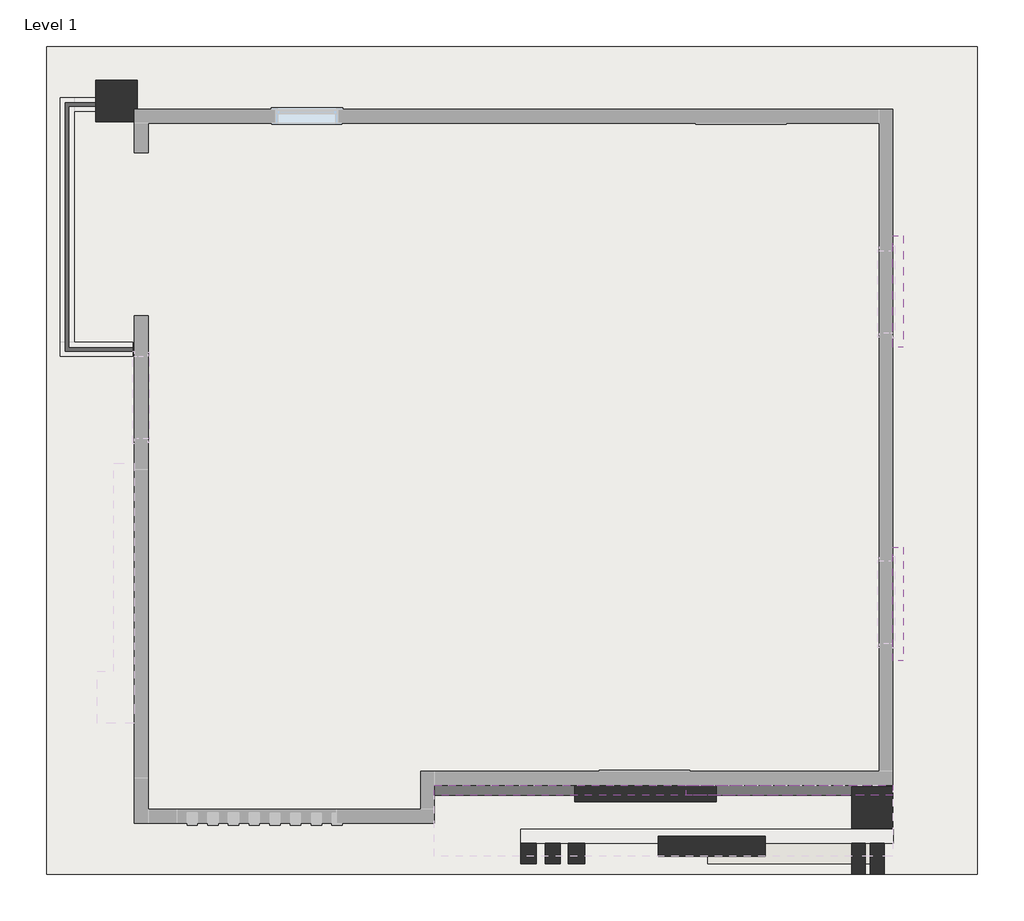
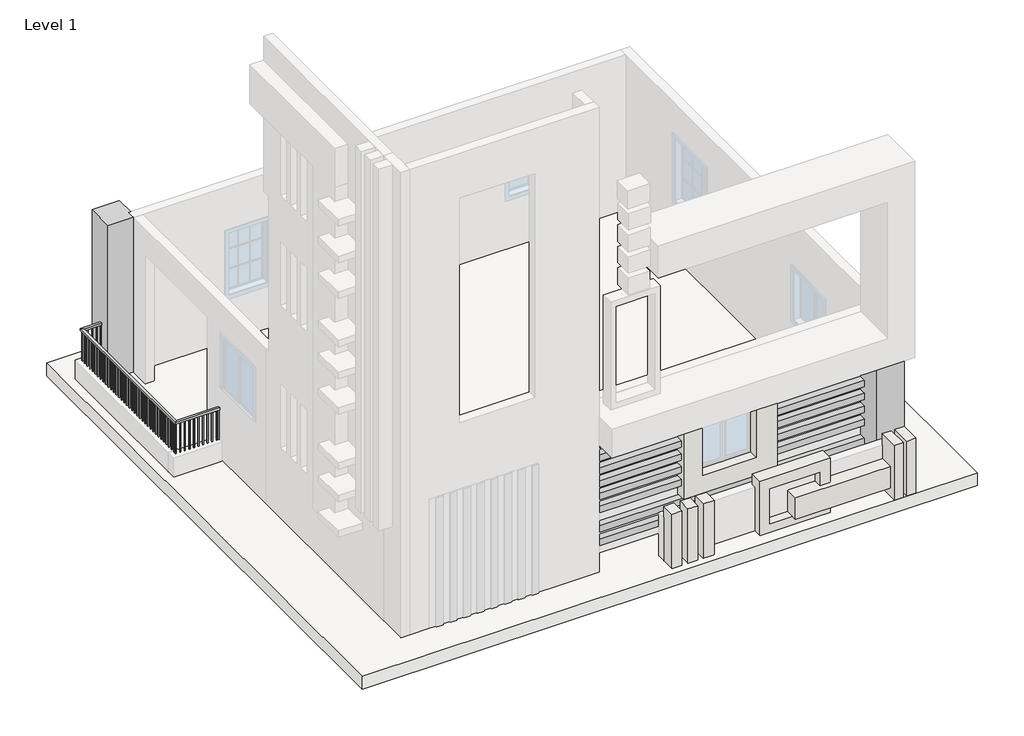
# One storey, part 2 of 2: 10 proxies, 2 columns, 2 walls, 1 railing, 1 slab.
"""IFC4 building model written with IfcOpenShell, lengths in millimetres."""

from ifc_helpers import new_model, si_unit, frame, origin, origin_with_axes, place, context, project, spatial, polyline, outline, extrude, faceted_brep, transform, mapped, element, save
from components import walls_6_walls_6_79d3fe83, walls_7_walls_7_e89f636e

model = new_model("IFC4")

# Units and contexts
model_context = context("Model", 3, world=origin())
ifc_project = project(units=[si_unit("LENGTHUNIT", "METRE", prefix="MILLI")], contexts=[model_context])

# Site, building, storey
site = spatial("IfcSite", under=ifc_project)
building = spatial("IfcBuilding", under=site)
storey = spatial("IfcBuildingStorey", under=building, Name="Level 1", Elevation=0.0)

# Proxies
placement = place(None, origin())
element("IfcBuildingElementProxy", 1, Name="Cornice", ObjectType="Cornice", at=placement, inside=storey, context=model_context, shape_type="SweptSolid", body=[
    extrude(outline(polyline([(-610.2932708, 6032.9483652), (-457.8932708, 6032.9483652), (-457.8932708, 4387.073901), (-610.2932708, 4387.073901), (-610.2932708, 6032.9483652)])), frame((0.0, 0.0, 2873.0721634), z_axis=(0.0, 0.0, 1.0), x_axis=(1.0, 0.0, 0.0)), (0.0, 0.0, 1.0), 152.4),
])
element("IfcBuildingElementProxy", 2, Name="Cornice", ObjectType="Cornice", at=placement, inside=storey, context=model_context, shape_type="SweptSolid", body=[
    extrude(outline(polyline([(-610.2932708, 1440.673901), (-457.8932708, 1440.673901), (-457.8932708, -235.726099), (-610.2932708, -235.726099), (-610.2932708, 1440.673901)])), frame((0.0, 0.0, 2594.4062448), z_axis=(0.0, 0.0, 1.0), x_axis=(1.0, 0.0, 0.0)), (0.0, 0.0, 1.0), 152.4),
    extrude(outline(polyline([(-610.2932708, 1440.673901), (-457.8932708, 1440.673901), (-457.8932708, -235.726099), (-610.2932708, -235.726099), (-610.2932708, 1440.673901)])), frame((0.0, 0.0, 2594.4062448), z_axis=(0.0, 0.0, 1.0), x_axis=(1.0, 0.0, 0.0)), (0.0, 0.0, 1.0), 152.4),
])
element("IfcBuildingElementProxy", 3, Name="Cornice", ObjectType="Cornice", at=placement, inside=storey, context=model_context, shape_type="SweptSolid", body=[
    extrude(outline(polyline([(-610.2932708, -2064.526099), (-610.2932708, -2216.926099), (-3658.2932708, -2216.926099), (-3658.2932708, -2064.526099), (-610.2932708, -2064.526099)])), frame((0.0, 0.0, 2286.0), z_axis=(0.0, 0.0, 1.0), x_axis=(1.0, 0.0, 0.0)), (0.0, 0.0, 1.0), 152.4),
    extrude(outline(polyline([(-4877.4932708, -2064.526099), (-4877.4932708, -2216.926099), (-7366.6932708, -2216.926099), (-7366.6932708, -2064.526099), (-4877.4932708, -2064.526099)])), frame((0.0, 0.0, 2286.0), z_axis=(0.0, 0.0, 1.0), x_axis=(1.0, 0.0, 0.0)), (0.0, 0.0, 1.0), 152.4),
])
element("IfcBuildingElementProxy", 4, Name="Cornice", ObjectType="Cornice", at=placement, inside=storey, context=model_context, shape_type="SweptSolid", body=[
    extrude(outline(polyline([(-610.2932708, -2064.526099), (-610.2932708, -2216.926099), (-3658.2932708, -2216.926099), (-3658.2932708, -2064.526099), (-610.2932708, -2064.526099)])), frame((0.0, 0.0, 1981.2), z_axis=(0.0, 0.0, 1.0), x_axis=(1.0, 0.0, 0.0)), (0.0, 0.0, 1.0), 152.4),
    extrude(outline(polyline([(-4877.4932708, -2064.526099), (-4877.4932708, -2216.926099), (-7366.6932708, -2216.926099), (-7366.6932708, -2064.526099), (-4877.4932708, -2064.526099)])), frame((0.0, 0.0, 1981.2), z_axis=(0.0, 0.0, 1.0), x_axis=(1.0, 0.0, 0.0)), (0.0, 0.0, 1.0), 152.4),
])
element("IfcBuildingElementProxy", 5, Name="Cornice", ObjectType="Cornice", at=placement, inside=storey, context=model_context, shape_type="SweptSolid", body=[
    extrude(outline(polyline([(-610.2932708, -2064.526099), (-610.2932708, -2216.926099), (-3658.2932708, -2216.926099), (-3658.2932708, -2064.526099), (-610.2932708, -2064.526099)])), frame((0.0, 0.0, 1676.4), z_axis=(0.0, 0.0, 1.0), x_axis=(1.0, 0.0, 0.0)), (0.0, 0.0, 1.0), 152.4),
    extrude(outline(polyline([(-4877.4932708, -2064.526099), (-4877.4932708, -2216.926099), (-7366.6932708, -2216.926099), (-7366.6932708, -2064.526099), (-4877.4932708, -2064.526099)])), frame((0.0, 0.0, 1676.4), z_axis=(0.0, 0.0, 1.0), x_axis=(1.0, 0.0, 0.0)), (0.0, 0.0, 1.0), 152.4),
])
element("IfcBuildingElementProxy", 6, Name="Cornice", ObjectType="Cornice", at=placement, inside=storey, context=model_context, shape_type="SweptSolid", body=[
    extrude(outline(polyline([(-610.2932708, -2064.526099), (-610.2932708, -2216.926099), (-7366.6932708, -2216.926099), (-7366.6932708, -2064.526099), (-610.2932708, -2064.526099)])), frame((0.0, 0.0, 2590.8), z_axis=(0.0, 0.0, 1.0), x_axis=(1.0, 0.0, 0.0)), (0.0, 0.0, 1.0), 152.4),
])
element("IfcBuildingElementProxy", 7, Name="Cornice", ObjectType="Cornice", at=placement, inside=storey, context=model_context, shape_type="SweptSolid", body=[
    extrude(outline(polyline([(-610.2932708, -2064.526099), (-610.2932708, -2216.926099), (-3658.2932708, -2216.926099), (-3658.2932708, -2064.526099), (-610.2932708, -2064.526099)])), frame((0.0, 0.0, 1371.6), z_axis=(0.0, 0.0, 1.0), x_axis=(1.0, 0.0, 0.0)), (0.0, 0.0, 1.0), 152.4),
    extrude(outline(polyline([(-4877.4932708, -2064.526099), (-4877.4932708, -2216.926099), (-7366.6932708, -2216.926099), (-7366.6932708, -2064.526099), (-4877.4932708, -2064.526099)])), frame((0.0, 0.0, 1371.6), z_axis=(0.0, 0.0, 1.0), x_axis=(1.0, 0.0, 0.0)), (0.0, 0.0, 1.0), 152.4),
])
element("IfcBuildingElementProxy", 8, Name="Cornice", ObjectType="Cornice", at=placement, inside=storey, context=model_context, shape_type="SweptSolid", body=[
    extrude(outline(polyline([(-610.2932708, -2064.526099), (-610.2932708, -2216.926099), (-7366.6932708, -2216.926099), (-7366.6932708, -2064.526099), (-610.2932708, -2064.526099)])), frame((0.0, 0.0, 1066.8), z_axis=(0.0, 0.0, 1.0), x_axis=(1.0, 0.0, 0.0)), (0.0, 0.0, 1.0), 152.4),
])
element("IfcBuildingElementProxy", 9, Name="Cornice", ObjectType="Cornice", at=placement, inside=storey, context=model_context, shape_type="SweptSolid", body=[
    extrude(outline(polyline([(-610.2932708, -2064.526099), (-610.2932708, -2216.926099), (-7366.6932708, -2216.926099), (-7366.6932708, -2064.526099), (-610.2932708, -2064.526099)])), frame((0.0, 0.0, 609.6), z_axis=(0.0, 0.0, 1.0), x_axis=(1.0, 0.0, 0.0)), (0.0, 0.0, 1.0), 152.4),
])
element("IfcBuildingElementProxy", 10, Name="Cornice", ObjectType="Cornice", at=placement, inside=storey, context=model_context, shape_type="SweptSolid", body=[
    extrude(outline(polyline([(-610.2932708, -2064.526099), (-610.2932708, -2216.926099), (-7366.6932708, -2216.926099), (-7366.6932708, -2064.526099), (-610.2932708, -2064.526099)])), frame((0.0, 0.0, 291.4800883), z_axis=(0.0, 0.0, 1.0), x_axis=(1.0, 0.0, 0.0)), (0.0, 0.0, 1.0), 152.4),
])

# Columns
element("IfcColumn", 11, ObjectType="Rectangular Column : 24\" x 24\"", at=placement, inside=storey, context=model_context, shape_type="Brep", body=[
    faceted_brep([(-11742.7083357, 8318.9483652, 3657.6), (-12352.3083357, 8318.9483652, 3657.6), (-12352.3083357, 7709.3483652, 3657.6), (-11786.2932708, 7709.3483652, 3657.6), (-11786.2932708, 7892.273901, 3657.6), (-11742.7083357, 7892.273901, 3657.6), (-12352.3083357, 7709.3483652, 0.0), (-12352.3083357, 7861.7483652, 0.0), (-12352.3083357, 8064.9483652, 0.0), (-12352.3083357, 8318.9483652, 0.0), (-11742.7083357, 8318.9483652, 0.0), (-11742.7083357, 7892.273901, 0.0), (-11786.2932708, 7892.273901, 0.0), (-11786.2932708, 7709.3483652, 0.0)], [[[0, 1, 2, 3, 4, 5]], [[6, 7, 8, 9, 10, 11, 12, 13]], [[1, 0, 10, 9]], [[2, 1, 9, 8, 7, 6]], [[2, 6, 13, 3]], [[10, 0, 5, 11]], [[4, 12, 11, 5]], [[12, 4, 3, 13]]]),
])
element("IfcColumn", 12, ObjectType="Rectangular Column : 24\" x 24\"", at=placement, inside=storey, context=model_context, shape_type="SweptSolid", body=[
    extrude(outline(polyline([(-610.2932708, -2089.926099), (-610.2932708, -2699.526099), (-1219.8932708, -2699.526099), (-1219.8932708, -2089.926099), (-610.2932708, -2089.926099)])), origin_with_axes(), (0.0, 0.0, 1.0), 3048.0),
])

# Railing
element("IfcRailing", 13, ObjectType="Handrail - Rectangular", at=placement, inside=storey, context=model_context, shape_type="SolidModel", body=[
    faceted_brep([(-12352.3083357, 7937.9483652, 1219.2), (-12352.3083357, 7937.9483652, 1168.4), (-12352.3083357, 7988.7483652, 1168.4), (-12352.3083357, 7988.7483652, 1219.2), (-12751.4932708, 7937.9483652, 1219.2), (-12751.4932708, 7937.9483652, 1168.4), (-12802.2932708, 7988.7483652, 1168.4), (-12802.2932708, 7988.7483652, 1219.2), (-12751.4932708, 4381.9483652, 1219.2), (-12751.4932708, 4381.9483652, 1168.4), (-12802.2932708, 4331.1483652, 1168.4), (-12802.2932708, 4331.1483652, 1219.2), (-11811.6932708, 4381.9483652, 1219.2), (-11811.6932708, 4331.1483652, 1219.2), (-11811.6932708, 4331.1483652, 1168.4), (-11811.6932708, 4381.9483652, 1168.4)], [[[0, 1, 2, 3]], [[1, 0, 4, 5]], [[2, 1, 5, 6]], [[3, 2, 6, 7]], [[0, 3, 7, 4]], [[5, 4, 8, 9]], [[6, 5, 9, 10]], [[7, 6, 10, 11]], [[4, 7, 11, 8]], [[12, 13, 14, 15]], [[9, 8, 12, 15]], [[10, 9, 15, 14]], [[11, 10, 14, 13]], [[8, 11, 13, 12]]]),
    extrude(outline(polyline([(-11872.0182708, 4347.0233652), (-11872.0182708, 4366.0733652), (-11852.9682708, 4366.0733652), (-11852.9682708, 4347.0233652), (-11872.0182708, 4347.0233652)])), frame((0.0, 0.0, 304.8), z_axis=(0.0, 0.0, 1.0), x_axis=(1.0, 0.0, 0.0)), (0.0, 0.0, 1.0), 863.6),
    extrude(outline(polyline([(-11973.6182708, 4347.0233652), (-11973.6182708, 4366.0733652), (-11954.5682708, 4366.0733652), (-11954.5682708, 4347.0233652), (-11973.6182708, 4347.0233652)])), frame((0.0, 0.0, 304.8), z_axis=(0.0, 0.0, 1.0), x_axis=(1.0, 0.0, 0.0)), (0.0, 0.0, 1.0), 863.6),
    extrude(outline(polyline([(-12075.2182708, 4347.0233652), (-12075.2182708, 4366.0733652), (-12056.1682708, 4366.0733652), (-12056.1682708, 4347.0233652), (-12075.2182708, 4347.0233652)])), frame((0.0, 0.0, 304.8), z_axis=(0.0, 0.0, 1.0), x_axis=(1.0, 0.0, 0.0)), (0.0, 0.0, 1.0), 863.6),
    extrude(outline(polyline([(-12176.8182708, 4347.0233652), (-12176.8182708, 4366.0733652), (-12157.7682708, 4366.0733652), (-12157.7682708, 4347.0233652), (-12176.8182708, 4347.0233652)])), frame((0.0, 0.0, 304.8), z_axis=(0.0, 0.0, 1.0), x_axis=(1.0, 0.0, 0.0)), (0.0, 0.0, 1.0), 863.6),
    extrude(outline(polyline([(-12278.4182708, 4347.0233652), (-12278.4182708, 4366.0733652), (-12259.3682708, 4366.0733652), (-12259.3682708, 4347.0233652), (-12278.4182708, 4347.0233652)])), frame((0.0, 0.0, 304.8), z_axis=(0.0, 0.0, 1.0), x_axis=(1.0, 0.0, 0.0)), (0.0, 0.0, 1.0), 863.6),
    extrude(outline(polyline([(-12380.0182708, 4347.0233652), (-12380.0182708, 4366.0733652), (-12360.9682708, 4366.0733652), (-12360.9682708, 4347.0233652), (-12380.0182708, 4347.0233652)])), frame((0.0, 0.0, 304.8), z_axis=(0.0, 0.0, 1.0), x_axis=(1.0, 0.0, 0.0)), (0.0, 0.0, 1.0), 863.6),
    extrude(outline(polyline([(-12481.6182708, 4347.0233652), (-12481.6182708, 4366.0733652), (-12462.5682708, 4366.0733652), (-12462.5682708, 4347.0233652), (-12481.6182708, 4347.0233652)])), frame((0.0, 0.0, 304.8), z_axis=(0.0, 0.0, 1.0), x_axis=(1.0, 0.0, 0.0)), (0.0, 0.0, 1.0), 863.6),
    extrude(outline(polyline([(-12583.2182708, 4347.0233652), (-12583.2182708, 4366.0733652), (-12564.1682708, 4366.0733652), (-12564.1682708, 4347.0233652), (-12583.2182708, 4347.0233652)])), frame((0.0, 0.0, 304.8), z_axis=(0.0, 0.0, 1.0), x_axis=(1.0, 0.0, 0.0)), (0.0, 0.0, 1.0), 863.6),
    extrude(outline(polyline([(-12684.8182708, 4347.0233652), (-12684.8182708, 4366.0733652), (-12665.7682708, 4366.0733652), (-12665.7682708, 4347.0233652), (-12684.8182708, 4347.0233652)])), frame((0.0, 0.0, 304.8), z_axis=(0.0, 0.0, 1.0), x_axis=(1.0, 0.0, 0.0)), (0.0, 0.0, 1.0), 863.6),
    extrude(outline(polyline([(-12786.4182708, 4416.8733652), (-12767.3682708, 4416.8733652), (-12767.3682708, 4397.8233652), (-12786.4182708, 4397.8233652), (-12786.4182708, 4416.8733652)])), frame((0.0, 0.0, 304.8), z_axis=(0.0, 0.0, 1.0), x_axis=(1.0, 0.0, 0.0)), (0.0, 0.0, 1.0), 863.6),
    extrude(outline(polyline([(-12786.4182708, 4518.4733652), (-12767.3682708, 4518.4733652), (-12767.3682708, 4499.4233652), (-12786.4182708, 4499.4233652), (-12786.4182708, 4518.4733652)])), frame((0.0, 0.0, 304.8), z_axis=(0.0, 0.0, 1.0), x_axis=(1.0, 0.0, 0.0)), (0.0, 0.0, 1.0), 863.6),
    extrude(outline(polyline([(-12786.4182708, 4620.0733652), (-12767.3682708, 4620.0733652), (-12767.3682708, 4601.0233652), (-12786.4182708, 4601.0233652), (-12786.4182708, 4620.0733652)])), frame((0.0, 0.0, 304.8), z_axis=(0.0, 0.0, 1.0), x_axis=(1.0, 0.0, 0.0)), (0.0, 0.0, 1.0), 863.6),
    extrude(outline(polyline([(-12786.4182708, 4721.6733652), (-12767.3682708, 4721.6733652), (-12767.3682708, 4702.6233652), (-12786.4182708, 4702.6233652), (-12786.4182708, 4721.6733652)])), frame((0.0, 0.0, 304.8), z_axis=(0.0, 0.0, 1.0), x_axis=(1.0, 0.0, 0.0)), (0.0, 0.0, 1.0), 863.6),
    extrude(outline(polyline([(-12786.4182708, 4823.2733652), (-12767.3682708, 4823.2733652), (-12767.3682708, 4804.2233652), (-12786.4182708, 4804.2233652), (-12786.4182708, 4823.2733652)])), frame((0.0, 0.0, 304.8), z_axis=(0.0, 0.0, 1.0), x_axis=(1.0, 0.0, 0.0)), (0.0, 0.0, 1.0), 863.6),
    extrude(outline(polyline([(-12786.4182708, 4924.8733652), (-12767.3682708, 4924.8733652), (-12767.3682708, 4905.8233652), (-12786.4182708, 4905.8233652), (-12786.4182708, 4924.8733652)])), frame((0.0, 0.0, 304.8), z_axis=(0.0, 0.0, 1.0), x_axis=(1.0, 0.0, 0.0)), (0.0, 0.0, 1.0), 863.6),
    extrude(outline(polyline([(-12786.4182708, 5026.4733652), (-12767.3682708, 5026.4733652), (-12767.3682708, 5007.4233652), (-12786.4182708, 5007.4233652), (-12786.4182708, 5026.4733652)])), frame((0.0, 0.0, 304.8), z_axis=(0.0, 0.0, 1.0), x_axis=(1.0, 0.0, 0.0)), (0.0, 0.0, 1.0), 863.6),
    extrude(outline(polyline([(-12786.4182708, 5128.0733652), (-12767.3682708, 5128.0733652), (-12767.3682708, 5109.0233652), (-12786.4182708, 5109.0233652), (-12786.4182708, 5128.0733652)])), frame((0.0, 0.0, 304.8), z_axis=(0.0, 0.0, 1.0), x_axis=(1.0, 0.0, 0.0)), (0.0, 0.0, 1.0), 863.6),
    extrude(outline(polyline([(-12786.4182708, 5229.6733652), (-12767.3682708, 5229.6733652), (-12767.3682708, 5210.6233652), (-12786.4182708, 5210.6233652), (-12786.4182708, 5229.6733652)])), frame((0.0, 0.0, 304.8), z_axis=(0.0, 0.0, 1.0), x_axis=(1.0, 0.0, 0.0)), (0.0, 0.0, 1.0), 863.6),
    extrude(outline(polyline([(-12786.4182708, 5331.2733652), (-12767.3682708, 5331.2733652), (-12767.3682708, 5312.2233652), (-12786.4182708, 5312.2233652), (-12786.4182708, 5331.2733652)])), frame((0.0, 0.0, 304.8), z_axis=(0.0, 0.0, 1.0), x_axis=(1.0, 0.0, 0.0)), (0.0, 0.0, 1.0), 863.6),
    extrude(outline(polyline([(-12786.4182708, 5432.8733652), (-12767.3682708, 5432.8733652), (-12767.3682708, 5413.8233652), (-12786.4182708, 5413.8233652), (-12786.4182708, 5432.8733652)])), frame((0.0, 0.0, 304.8), z_axis=(0.0, 0.0, 1.0), x_axis=(1.0, 0.0, 0.0)), (0.0, 0.0, 1.0), 863.6),
    extrude(outline(polyline([(-12786.4182708, 5534.4733652), (-12767.3682708, 5534.4733652), (-12767.3682708, 5515.4233652), (-12786.4182708, 5515.4233652), (-12786.4182708, 5534.4733652)])), frame((0.0, 0.0, 304.8), z_axis=(0.0, 0.0, 1.0), x_axis=(1.0, 0.0, 0.0)), (0.0, 0.0, 1.0), 863.6),
    extrude(outline(polyline([(-12786.4182708, 5636.0733652), (-12767.3682708, 5636.0733652), (-12767.3682708, 5617.0233652), (-12786.4182708, 5617.0233652), (-12786.4182708, 5636.0733652)])), frame((0.0, 0.0, 304.8), z_axis=(0.0, 0.0, 1.0), x_axis=(1.0, 0.0, 0.0)), (0.0, 0.0, 1.0), 863.6),
    extrude(outline(polyline([(-12786.4182708, 5737.6733652), (-12767.3682708, 5737.6733652), (-12767.3682708, 5718.6233652), (-12786.4182708, 5718.6233652), (-12786.4182708, 5737.6733652)])), frame((0.0, 0.0, 304.8), z_axis=(0.0, 0.0, 1.0), x_axis=(1.0, 0.0, 0.0)), (0.0, 0.0, 1.0), 863.6),
    extrude(outline(polyline([(-12786.4182708, 5839.2733652), (-12767.3682708, 5839.2733652), (-12767.3682708, 5820.2233652), (-12786.4182708, 5820.2233652), (-12786.4182708, 5839.2733652)])), frame((0.0, 0.0, 304.8), z_axis=(0.0, 0.0, 1.0), x_axis=(1.0, 0.0, 0.0)), (0.0, 0.0, 1.0), 863.6),
    extrude(outline(polyline([(-12786.4182708, 5940.8733652), (-12767.3682708, 5940.8733652), (-12767.3682708, 5921.8233652), (-12786.4182708, 5921.8233652), (-12786.4182708, 5940.8733652)])), frame((0.0, 0.0, 304.8), z_axis=(0.0, 0.0, 1.0), x_axis=(1.0, 0.0, 0.0)), (0.0, 0.0, 1.0), 863.6),
    extrude(outline(polyline([(-12786.4182708, 6042.4733652), (-12767.3682708, 6042.4733652), (-12767.3682708, 6023.4233652), (-12786.4182708, 6023.4233652), (-12786.4182708, 6042.4733652)])), frame((0.0, 0.0, 304.8), z_axis=(0.0, 0.0, 1.0), x_axis=(1.0, 0.0, 0.0)), (0.0, 0.0, 1.0), 863.6),
    extrude(outline(polyline([(-12786.4182708, 6144.0733652), (-12767.3682708, 6144.0733652), (-12767.3682708, 6125.0233652), (-12786.4182708, 6125.0233652), (-12786.4182708, 6144.0733652)])), frame((0.0, 0.0, 304.8), z_axis=(0.0, 0.0, 1.0), x_axis=(1.0, 0.0, 0.0)), (0.0, 0.0, 1.0), 863.6),
    extrude(outline(polyline([(-12786.4182708, 6245.6733652), (-12767.3682708, 6245.6733652), (-12767.3682708, 6226.6233652), (-12786.4182708, 6226.6233652), (-12786.4182708, 6245.6733652)])), frame((0.0, 0.0, 304.8), z_axis=(0.0, 0.0, 1.0), x_axis=(1.0, 0.0, 0.0)), (0.0, 0.0, 1.0), 863.6),
    extrude(outline(polyline([(-12786.4182708, 6347.2733652), (-12767.3682708, 6347.2733652), (-12767.3682708, 6328.2233652), (-12786.4182708, 6328.2233652), (-12786.4182708, 6347.2733652)])), frame((0.0, 0.0, 304.8), z_axis=(0.0, 0.0, 1.0), x_axis=(1.0, 0.0, 0.0)), (0.0, 0.0, 1.0), 863.6),
    extrude(outline(polyline([(-12786.4182708, 6448.8733652), (-12767.3682708, 6448.8733652), (-12767.3682708, 6429.8233652), (-12786.4182708, 6429.8233652), (-12786.4182708, 6448.8733652)])), frame((0.0, 0.0, 304.8), z_axis=(0.0, 0.0, 1.0), x_axis=(1.0, 0.0, 0.0)), (0.0, 0.0, 1.0), 863.6),
    extrude(outline(polyline([(-12786.4182708, 6550.4733652), (-12767.3682708, 6550.4733652), (-12767.3682708, 6531.4233652), (-12786.4182708, 6531.4233652), (-12786.4182708, 6550.4733652)])), frame((0.0, 0.0, 304.8), z_axis=(0.0, 0.0, 1.0), x_axis=(1.0, 0.0, 0.0)), (0.0, 0.0, 1.0), 863.6),
    extrude(outline(polyline([(-12786.4182708, 6652.0733652), (-12767.3682708, 6652.0733652), (-12767.3682708, 6633.0233652), (-12786.4182708, 6633.0233652), (-12786.4182708, 6652.0733652)])), frame((0.0, 0.0, 304.8), z_axis=(0.0, 0.0, 1.0), x_axis=(1.0, 0.0, 0.0)), (0.0, 0.0, 1.0), 863.6),
    extrude(outline(polyline([(-12786.4182708, 6753.6733652), (-12767.3682708, 6753.6733652), (-12767.3682708, 6734.6233652), (-12786.4182708, 6734.6233652), (-12786.4182708, 6753.6733652)])), frame((0.0, 0.0, 304.8), z_axis=(0.0, 0.0, 1.0), x_axis=(1.0, 0.0, 0.0)), (0.0, 0.0, 1.0), 863.6),
    extrude(outline(polyline([(-12786.4182708, 6855.2733652), (-12767.3682708, 6855.2733652), (-12767.3682708, 6836.2233652), (-12786.4182708, 6836.2233652), (-12786.4182708, 6855.2733652)])), frame((0.0, 0.0, 304.8), z_axis=(0.0, 0.0, 1.0), x_axis=(1.0, 0.0, 0.0)), (0.0, 0.0, 1.0), 863.6),
    extrude(outline(polyline([(-12786.4182708, 6956.8733652), (-12767.3682708, 6956.8733652), (-12767.3682708, 6937.8233652), (-12786.4182708, 6937.8233652), (-12786.4182708, 6956.8733652)])), frame((0.0, 0.0, 304.8), z_axis=(0.0, 0.0, 1.0), x_axis=(1.0, 0.0, 0.0)), (0.0, 0.0, 1.0), 863.6),
    extrude(outline(polyline([(-12786.4182708, 7058.4733652), (-12767.3682708, 7058.4733652), (-12767.3682708, 7039.4233652), (-12786.4182708, 7039.4233652), (-12786.4182708, 7058.4733652)])), frame((0.0, 0.0, 304.8), z_axis=(0.0, 0.0, 1.0), x_axis=(1.0, 0.0, 0.0)), (0.0, 0.0, 1.0), 863.6),
    extrude(outline(polyline([(-12786.4182708, 7160.0733652), (-12767.3682708, 7160.0733652), (-12767.3682708, 7141.0233652), (-12786.4182708, 7141.0233652), (-12786.4182708, 7160.0733652)])), frame((0.0, 0.0, 304.8), z_axis=(0.0, 0.0, 1.0), x_axis=(1.0, 0.0, 0.0)), (0.0, 0.0, 1.0), 863.6),
    extrude(outline(polyline([(-12786.4182708, 7261.6733652), (-12767.3682708, 7261.6733652), (-12767.3682708, 7242.6233652), (-12786.4182708, 7242.6233652), (-12786.4182708, 7261.6733652)])), frame((0.0, 0.0, 304.8), z_axis=(0.0, 0.0, 1.0), x_axis=(1.0, 0.0, 0.0)), (0.0, 0.0, 1.0), 863.6),
    extrude(outline(polyline([(-12786.4182708, 7363.2733652), (-12767.3682708, 7363.2733652), (-12767.3682708, 7344.2233652), (-12786.4182708, 7344.2233652), (-12786.4182708, 7363.2733652)])), frame((0.0, 0.0, 304.8), z_axis=(0.0, 0.0, 1.0), x_axis=(1.0, 0.0, 0.0)), (0.0, 0.0, 1.0), 863.6),
    extrude(outline(polyline([(-12786.4182708, 7464.8733652), (-12767.3682708, 7464.8733652), (-12767.3682708, 7445.8233652), (-12786.4182708, 7445.8233652), (-12786.4182708, 7464.8733652)])), frame((0.0, 0.0, 304.8), z_axis=(0.0, 0.0, 1.0), x_axis=(1.0, 0.0, 0.0)), (0.0, 0.0, 1.0), 863.6),
    extrude(outline(polyline([(-12786.4182708, 7566.4733652), (-12767.3682708, 7566.4733652), (-12767.3682708, 7547.4233652), (-12786.4182708, 7547.4233652), (-12786.4182708, 7566.4733652)])), frame((0.0, 0.0, 304.8), z_axis=(0.0, 0.0, 1.0), x_axis=(1.0, 0.0, 0.0)), (0.0, 0.0, 1.0), 863.6),
    extrude(outline(polyline([(-12786.4182708, 7668.0733652), (-12767.3682708, 7668.0733652), (-12767.3682708, 7649.0233652), (-12786.4182708, 7649.0233652), (-12786.4182708, 7668.0733652)])), frame((0.0, 0.0, 304.8), z_axis=(0.0, 0.0, 1.0), x_axis=(1.0, 0.0, 0.0)), (0.0, 0.0, 1.0), 863.6),
    extrude(outline(polyline([(-12786.4182708, 7769.6733652), (-12767.3682708, 7769.6733652), (-12767.3682708, 7750.6233652), (-12786.4182708, 7750.6233652), (-12786.4182708, 7769.6733652)])), frame((0.0, 0.0, 304.8), z_axis=(0.0, 0.0, 1.0), x_axis=(1.0, 0.0, 0.0)), (0.0, 0.0, 1.0), 863.6),
    extrude(outline(polyline([(-12786.4182708, 7871.2733652), (-12767.3682708, 7871.2733652), (-12767.3682708, 7852.2233652), (-12786.4182708, 7852.2233652), (-12786.4182708, 7871.2733652)])), frame((0.0, 0.0, 304.8), z_axis=(0.0, 0.0, 1.0), x_axis=(1.0, 0.0, 0.0)), (0.0, 0.0, 1.0), 863.6),
    extrude(outline(polyline([(-12749.1833357, 7972.8733652), (-12749.1833357, 7953.8233652), (-12768.2333357, 7953.8233652), (-12768.2333357, 7972.8733652), (-12749.1833357, 7972.8733652)])), frame((0.0, 0.0, 304.8), z_axis=(0.0, 0.0, 1.0), x_axis=(1.0, 0.0, 0.0)), (0.0, 0.0, 1.0), 863.6),
    extrude(outline(polyline([(-12647.5833357, 7972.8733652), (-12647.5833357, 7953.8233652), (-12666.6333357, 7953.8233652), (-12666.6333357, 7972.8733652), (-12647.5833357, 7972.8733652)])), frame((0.0, 0.0, 304.8), z_axis=(0.0, 0.0, 1.0), x_axis=(1.0, 0.0, 0.0)), (0.0, 0.0, 1.0), 863.6),
    extrude(outline(polyline([(-12545.9833357, 7972.8733652), (-12545.9833357, 7953.8233652), (-12565.0333357, 7953.8233652), (-12565.0333357, 7972.8733652), (-12545.9833357, 7972.8733652)])), frame((0.0, 0.0, 304.8), z_axis=(0.0, 0.0, 1.0), x_axis=(1.0, 0.0, 0.0)), (0.0, 0.0, 1.0), 863.6),
    extrude(outline(polyline([(-12444.3833357, 7972.8733652), (-12444.3833357, 7953.8233652), (-12463.4333357, 7953.8233652), (-12463.4333357, 7972.8733652), (-12444.3833357, 7972.8733652)])), frame((0.0, 0.0, 304.8), z_axis=(0.0, 0.0, 1.0), x_axis=(1.0, 0.0, 0.0)), (0.0, 0.0, 1.0), 863.6),
    extrude(outline(polyline([(-12786.4182708, 4366.0733652), (-12767.3682708, 4366.0733652), (-12767.3682708, 4347.0233652), (-12786.4182708, 4347.0233652), (-12786.4182708, 4366.0733652)])), frame((0.0, 0.0, 304.8), z_axis=(0.0, 0.0, 1.0), x_axis=(1.0, 0.0, 0.0)), (0.0, 0.0, 1.0), 863.6),
    extrude(outline(polyline([(-12767.3682708, 7972.8733652), (-12767.3682708, 7953.8233652), (-12786.4182708, 7953.8233652), (-12786.4182708, 7972.8733652), (-12767.3682708, 7972.8733652)])), frame((0.0, 0.0, 304.8), z_axis=(0.0, 0.0, 1.0), x_axis=(1.0, 0.0, 0.0)), (0.0, 0.0, 1.0), 863.6),
    extrude(outline(polyline([(-11830.7432708, 4347.0233652), (-11830.7432708, 4366.0733652), (-11811.6932708, 4366.0733652), (-11811.6932708, 4347.0233652), (-11830.7432708, 4347.0233652)])), frame((0.0, 0.0, 304.8), z_axis=(0.0, 0.0, 1.0), x_axis=(1.0, 0.0, 0.0)), (0.0, 0.0, 1.0), 863.6),
    extrude(outline(polyline([(-12352.3083357, 7972.8733652), (-12352.3083357, 7953.8233652), (-12371.3583357, 7953.8233652), (-12371.3583357, 7972.8733652), (-12352.3083357, 7972.8733652)])), frame((0.0, 0.0, 304.8), z_axis=(0.0, 0.0, 1.0), x_axis=(1.0, 0.0, 0.0)), (0.0, 0.0, 1.0), 863.6),
])

# Slab
element("IfcSlab", 14, ObjectType="Generic - 12\"", at=placement, inside=storey, context=model_context, shape_type="SweptSolid", body=[
    extrude(outline(polyline([(635.4256217, 8817.5737668), (635.4256217, -3374.4262332), (-13080.5743783, -3374.4262332), (-13080.5743783, 8817.5737668), (635.4256217, 8817.5737668)])), frame((0.0, 0.0, -304.8), z_axis=(0.0, 0.0, 1.0), x_axis=(1.0, 0.0, 0.0)), (0.0, 0.0, 1.0), 304.8),
])

# Walls
walls_6_walls_6_shape = walls_6_walls_6_79d3fe83(model_context)
element("IfcWall", 15, ObjectType="Walls 6 : Walls 6", at=placement, inside=storey, context=model_context, shape_type="MappedRepresentation", body=[
    mapped(walls_6_walls_6_shape, transform((0.0, 0.0, 0.0), x_axis=(1.0, 0.0, 0.0), y_axis=(0.0, 1.0, 0.0), z_axis=(0.0, 0.0, 1.0))),
])
walls_7_walls_7_shape = walls_7_walls_7_e89f636e(model_context)
element("IfcWall", 16, ObjectType="Walls 7 : Walls 7", at=placement, inside=storey, context=model_context, shape_type="MappedRepresentation", body=[
    mapped(walls_7_walls_7_shape, transform((0.0, 0.0, 0.0), x_axis=(1.0, 0.0, 0.0), y_axis=(0.0, 1.0, 0.0), z_axis=(0.0, 0.0, 1.0))),
])

save(model, "model.ifc")

# Revit data of these elements
# Type "Rectangular Column : 24\" x 24\""
#   Assembly Code = "B1010200"
#   Depth = 2' - 0"
#   Offset Base = 0' - 0"
#   Offset Top = 0' - 0"
#   Width = 2' - 0"
#   Material = none
# Type "Handrail - Rectangular"
#   Assembly Code = "C2010400"
#   built-in parameter 1008612 = 0.0416667 (stored number, unit not read)
#   built-in parameter 1008611 = 0.0416667 (stored number, unit not read)
#   built-in parameter 1008609 = 0.333333 (stored number, unit not read)
#   built-in parameter 1008604 = 0.166667 (stored number, unit not read)
#   built-in parameter 1008603 = 0.166667 (stored number, unit not read)
#   Railing Height = 3' - 0"
#   built-in parameter 1008630 = 2
#   built-in parameter 1008610 = 2
#   built-in parameter 1008618 = Baluster - Square : 3/4"
# Type "Generic - 12\""
#   Assembly Code = "B1010"
#   Function = 0
#   Layers, outside or top first: 1' - 0" no material (function 1)
# Elements 1, 2, 3, 4, 5, 6, 7, 8, 9, 10 (IfcBuildingElementProxy, "Cornice")
#   Phase Created = New Construction
#   Materials on its faces: "Default Wall"
# Element 11 (IfcColumn, "Rectangular Column : 24\" x 24\"")
#   Phase Created = New Construction
#   Materials on its faces: "Default Wall"
# Element 12 (IfcColumn, "Rectangular Column : 24\" x 24\"")
#   Phase Created = New Construction
# Element 13 (IfcRailing, "Handrail - Rectangular")
#   built-in parameter 1008621 = 1 (stored number, unit not read)
#   Phase Created = New Construction
# Element 14 (IfcSlab, "Generic - 12\"")
#   Height Offset From Level = 0' - 0"
#   Phase Created = New Construction
#   Materials on its faces: "Default Floor"
# Element 15 (IfcWall, "Walls 6 : Walls 6")
#   Phase Created = New Construction
#   Materials on its faces: "Default Wall"
# Element 16 (IfcWall, "Walls 7 : Walls 7")
#   Phase Created = New Construction
#   Materials on its faces: "Default Wall"
# Materials
#   "Default Wall": colour RGB 128 128 128, transparency 0
#   "Default Floor": colour RGB 128 128 128, transparency 0
